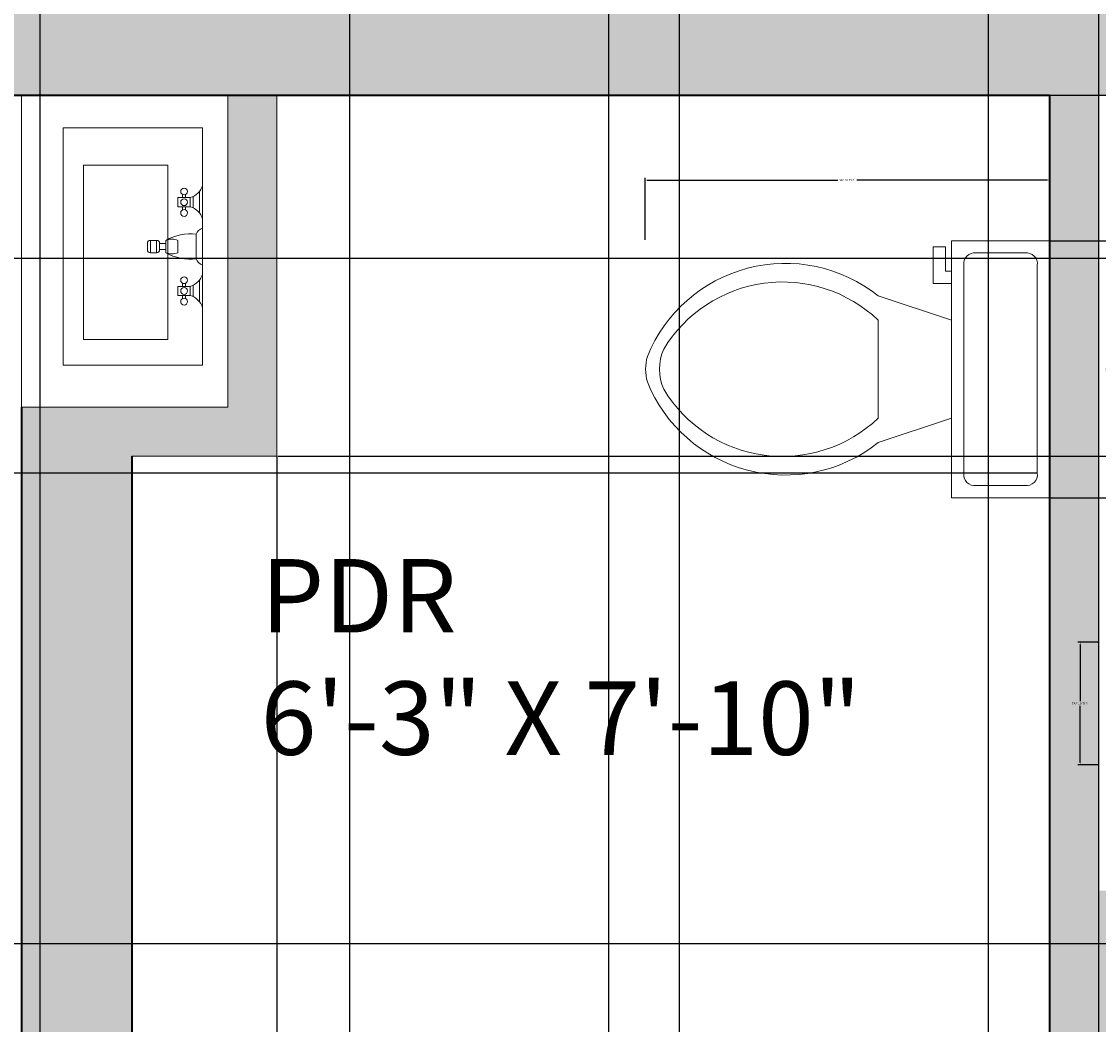
# Model space of a CAD drawing. Units: inches. Extents: x 818 to 1898, y 976 to 2364.
# Tile 51 of 96: x 1512 to 1600, y 1791 to 1873. Entities that reach past the tile are written whole.
import ezdxf

# ---------------------------------------------------------------- set-up
doc = ezdxf.new("R2010")
doc.units = ezdxf.units.IN
doc.header["$LTSCALE"] = 5
doc.header["$MEASUREMENT"] = 0
for name, color, linetype, lineweight in [('A-ANNO-DIMS', 2, 'Continuous', 18), ('A-AREA-IDEN', 7, 'Continuous', 18), ('A-FLOR-FIXT', 9, 'Continuous', 18), ('A-WALL', 7, 'Continuous', 40)]:
    doc.layers.add(name, color=color, linetype=linetype, lineweight=lineweight)
doc.layers.add('A-WALL-PATT', color=251, linetype='Continuous', lineweight=13, true_color=0x636466)
doc.styles.get("Standard").update_dxf_attribs({"font": 'arial.ttf'})
doc.dimstyles.get("Standard").update_dxf_attribs({"dimtxt": 0.18, "dimasz": 0.18, "dimexe": 0.18, "dimexo": 0.0625, "dimgap": 0.09, "dimtad": 0, "dimtih": 1, "dimtoh": 1, "dimdec": 4, "dimzin": 0, "dimdsep": 46, "dimtxsty": 'Standard', "dimcen": 0.09, "dimadec": 0, "dimazin": 0, "dimtfac": 1, "dimtdec": 4, "dimtofl": 0, "dimtmove": 0, "dimatfit": 3, "dimfxl": 1, "dimtolj": 1, "dimtzin": 0, "dimarcsym": 0})

# ---------------------------------------------------------------- blocks, each defined once
blk = doc.blocks.new('Toilet - top')
for p, q in [((9.5, -6), (9.5, -2)), ((-10, -8.5), (-8, -8.5)), ((-10, -9.5), (-10, -8.5)), ((-8, -8.5), (-8, -8)), ((-7, -8), (-7, -9.5)), ((-4, -8), (-6, -14)), ((4, -8), (6, -14)), ((-7, -9.5), (-10, -9.5)), ((4, -14), (-4, -14))]:
    blk.add_line(p, q)
blk.add_lwpolyline([(10.5, -8), (10.5, 0), (-10.5, 0), (-10.5, -8)], close=True)
for points in [[(8.5, -1), (-8.5, -1)], [(-9.5, -2), (-9.5, -6)], [(-8.5, -7), (8.5, -7)]]:
    blk.add_lwpolyline(points)
for centre, radius, start, end in [((-8.625, -1.875), 0.884, 81.8699, 188.1301), ((8.625, -1.875), 0.884, 351.8699, 98.1301), ((-8.625, -6.125), 0.884, 171.8699, 278.1301), ((8.625, -6.125), 0.884, 261.8699, 8.1301), ((3.52, -21.58), 12.169, 141.46911, 247.97143), ((4.2, -21.817), 11.329, 136.36773, 238.94682), ((-3.519, -21.58), 12.169, 292.02843, 38.53071), ((-4.2, -21.817), 11.329, 301.05301, 43.63209), ((0, -27.876), 4, 245.73182, 294.26817), ((0, -29), 4, 254.86053, 285.13947)]:
    blk.add_arc(centre, radius, start, end)
blk = doc.blocks.new('Faucet - Bathroom front')
for p, q in [((-0.5, 4.25), (0.5, 4.25)), ((0.5, 3.75), (-0.5, 3.75)), ((-0.5, 3), (0.5, 3)), ((-0.25, 3), (-0.25, 3.5)), ((0.25, 3.5), (0.25, 3)), ((0.5, 2), (-0.5, 2)), ((-4, 1.625), (-4.25, 1.625)), ((-4, 1.375), (-4.25, 1.375)), ((-3.25, 1.625), (-3, 1.625)), ((-3.25, 1.375), (-3, 1.375)), ((3.25, 1.625), (3, 1.625)), ((3.25, 1.375), (3, 1.375)), ((4, 1.625), (4.25, 1.625)), ((4, 1.375), (4.25, 1.375)), ((-5, 0), (-2.25, 0)), ((-4.5087, 0.25), (-2.7408, 0.25)), ((-3.1442, 0.75), (-4.0979, 0.75)), ((-1.5, 0), (1.5, 0)), ((-1, 0.5), (1, 0.5)), ((2.25, 0), (5, 0)), ((2.7413, 0.25), (4.5092, 0.25)), ((4.1058, 0.75), (3.1521, 0.75))]:
    blk.add_line(p, q)
for points in [[(-0.25, 4.5), (0.25, 4.5)], [(-0.5, 3.75), (-0.5, 4.25)], [(0.5, 4.25), (0.5, 3.75)], [(0.25, 3.5), (-0.25, 3.5)]]:
    blk.add_lwpolyline(points)
for points in [[(-4, 1), (-4, 2), (-3.25, 2), (-3.25, 1)], [(3.25, 1), (3.25, 2), (4, 2), (4, 1)]]:
    blk.add_lwpolyline(points, close=True)
for centre in [(-4.5, 1.5), (-3.625, 1.5), (-2.75, 1.5), (2.75, 1.5), (3.625, 1.5), (4.5, 1.5)]:
    blk.add_circle(centre, 0.2795)
for centre, radius, start, end in [((-0.2575, 4.2575), 0.2426, 88.22243, 181.7776), ((0.2575, 4.2575), 0.2426, 358.2224, 91.77757), ((-0.2575, 3.7425), 0.2426, 178.2224, 271.7776), ((0.2575, 3.7425), 0.2426, 268.2224, 1.777565), ((3, 1), 4.0311, 150.2551, 187.125), ((0.6413, 2.5), 1.246, 156.3417, 203.6583), ((-3, 1), 4.0311, 352.875, 29.74488), ((-0.6413, 2.5), 1.246, 336.3417, 23.65835), ((-5.375, 1.375), 1.4252, 285.2551, 344.7449), ((-1.875, 1.375), 1.4252, 195.2551, 254.7449), ((1.875, 1.375), 1.4252, 285.2551, 344.7449), ((5.375, 1.375), 1.4252, 195.2551, 254.7449), ((-0.7962, -0.2038), 0.7327, 106.1502, 163.8498), ((0.7962, -0.2038), 0.7327, 16.1502, 73.84979)]:
    blk.add_arc(centre, radius, start, end)
blk = doc.blocks.new('*D36')
at = {"layer": 'A-ANNO-DIMS', "color": 0, "lineweight": -2, "ltscale": 5, "transparency": 16777216}
for p, q in [((1599.663, 1822.366), (1598.045, 1822.366)), ((1598.225, 1822.186), (1598.225, 1817.548)), ((1598.225, 1812.546), (1598.225, 1817.184)), ((1599.663, 1812.366), (1598.045, 1812.366))]:
    blk.add_line(p, q, dxfattribs=at)
at = {"layer": 'A-ANNO-DIMS', "color": 0, "ltscale": 5, "transparency": 16777216}
for points in [[(1598.195, 1822.186), (1598.255, 1822.186), (1598.225, 1822.366)], [(1598.195, 1812.546), (1598.255, 1812.546), (1598.225, 1812.366)]]:
    blk.add_solid(points, dxfattribs=at)
at = {"layer": 'Defpoints', "color": 0, "ltscale": 5, "transparency": 16777216}
for p in [(1599.725, 1822.366), (1598.225, 1812.366), (1599.725, 1812.366)]:
    blk.add_point(p, dxfattribs=at)
at = {"layer": 'A-ANNO-DIMS', "color": 0, "ltscale": 5, "transparency": 16777216, "insert": (1598.225, 1817.366), "char_height": 0.18, "attachment_point": 5}
blk.add_mtext('\\A1;TAP 10 TYP.', dxfattribs=at)
blk = doc.blocks.new('*D40')
at = {"layer": 'A-ANNO-DIMS', "color": 0, "lineweight": -2, "ltscale": 5, "transparency": 16777216}
for p, q in [((1562.679, 1855.247), (1562.679, 1860.321)), ((1595.725, 1855.247), (1595.725, 1860.321)), ((1562.859, 1860.141), (1578.426, 1860.141)), ((1595.545, 1860.141), (1579.978, 1860.141))]:
    blk.add_line(p, q, dxfattribs=at)
at = {"layer": 'A-ANNO-DIMS', "color": 0, "ltscale": 5, "transparency": 16777216}
for points in [[(1562.859, 1860.171), (1562.859, 1860.111), (1562.679, 1860.141)], [(1595.545, 1860.171), (1595.545, 1860.111), (1595.725, 1860.141)]]:
    blk.add_solid(points, dxfattribs=at)
at = {"layer": 'Defpoints', "color": 0, "ltscale": 5, "transparency": 16777216}
for p in [(1595.725, 1860.141), (1562.679, 1855.184), (1595.725, 1855.184)]:
    blk.add_point(p, dxfattribs=at)
at = {"layer": 'A-ANNO-DIMS', "color": 0, "ltscale": 5, "transparency": 16777216, "insert": (1579.202, 1860.141), "char_height": 0.18, "attachment_point": 5}
blk.add_mtext('\\A1;WC 33 TYP.', dxfattribs=at)
blk = doc.blocks.new('*D41')
at = {"layer": 'A-ANNO-DIMS', "color": 0, "lineweight": -2, "ltscale": 5, "transparency": 16777216}
for p, q in [((1595.788, 1855.184), (1600.862, 1855.184)), ((1600.682, 1855.004), (1600.682, 1844.865)), ((1600.682, 1834.364), (1600.682, 1844.504)), ((1595.788, 1834.184), (1600.862, 1834.184))]:
    blk.add_line(p, q, dxfattribs=at)
at = {"layer": 'A-ANNO-DIMS', "color": 0, "ltscale": 5, "transparency": 16777216}
for points in [[(1600.652, 1855.004), (1600.712, 1855.004), (1600.682, 1855.184)], [(1600.652, 1834.364), (1600.712, 1834.364), (1600.682, 1834.184)]]:
    blk.add_solid(points, dxfattribs=at)
at = {"layer": 'Defpoints', "color": 0, "ltscale": 5, "transparency": 16777216}
for p in [(1595.725, 1855.184), (1595.725, 1834.184), (1600.682, 1834.184)]:
    blk.add_point(p, dxfattribs=at)
at = {"layer": 'A-ANNO-DIMS', "color": 0, "ltscale": 5, "transparency": 16777216, "insert": (1600.682, 1844.684), "char_height": 0.18, "attachment_point": 5}
blk.add_mtext('\\A1;21 TYP.', dxfattribs=at)
blk = doc.blocks.new('*D85')
at = {"layer": 'A-ANNO-DIMS', "color": 0, "lineweight": -2, "ltscale": 5, "transparency": 16777216}
for p, q in [((1258.788, 2053.078), (1897.916, 2053.078)), ((1897.736, 2052.898), (1897.736, 1876.76)), ((1897.736, 1700.258), (1897.736, 1876.396)), ((1258.788, 1700.078), (1897.916, 1700.078))]:
    blk.add_line(p, q, dxfattribs=at)
at = {"layer": 'A-ANNO-DIMS', "color": 0, "ltscale": 5, "transparency": 16777216}
for points in [[(1897.706, 2052.898), (1897.766, 2052.898), (1897.736, 2053.078)], [(1897.706, 1700.258), (1897.766, 1700.258), (1897.736, 1700.078)]]:
    blk.add_solid(points, dxfattribs=at)
at = {"layer": 'Defpoints', "color": 0, "ltscale": 5, "transparency": 16777216}
for p in [(1258.725, 2053.078), (1897.736, 2053.078), (1258.725, 1700.078)]:
    blk.add_point(p, dxfattribs=at)
at = {"layer": 'A-ANNO-DIMS', "color": 0, "ltscale": 5, "transparency": 16777216, "insert": (1897.736, 1876.578), "char_height": 0.18, "attachment_point": 5}
blk.add_mtext('\\A1;353', dxfattribs=at)
blk = doc.blocks.new('*D101')
at = {"layer": 'A-ANNO-DIMS', "color": 0, "lineweight": -2, "ltscale": 5, "transparency": 16777216}
for p, q in [((1507.298, 1071.118), (1507.298, 2363.873)), ((1507.478, 2363.693), (1535.997, 2363.693)), ((1565.303, 2363.693), (1536.785, 2363.693)), ((1565.483, 1071.118), (1565.483, 2363.873))]:
    blk.add_line(p, q, dxfattribs=at)
at = {"layer": 'A-ANNO-DIMS', "color": 0, "ltscale": 5, "transparency": 16777216}
for points in [[(1507.478, 2363.723), (1507.478, 2363.663), (1507.298, 2363.693)], [(1565.303, 2363.723), (1565.303, 2363.663), (1565.483, 2363.693)]]:
    blk.add_solid(points, dxfattribs=at)
at = {"layer": 'Defpoints', "color": 0, "ltscale": 5, "transparency": 16777216}
for p in [(1565.483, 2363.693), (1507.298, 1071.055), (1565.483, 1071.055)]:
    blk.add_point(p, dxfattribs=at)
at = {"layer": 'A-ANNO-DIMS', "color": 0, "ltscale": 5, "transparency": 16777216, "insert": (1536.391, 2363.693), "char_height": 0.18, "attachment_point": 5}
blk.add_mtext('\\A1;58.19', dxfattribs=at)
blk = doc.blocks.new('*D102')
at = {"layer": 'A-ANNO-DIMS', "color": 0, "lineweight": -2, "ltscale": 5, "transparency": 16777216}
for p, q in [((1565.483, 1071.118), (1565.483, 2363.873)), ((1565.663, 2363.693), (1595.635, 2363.693)), ((1626.395, 2363.693), (1596.423, 2363.693)), ((1626.575, 1071.118), (1626.575, 2363.873))]:
    blk.add_line(p, q, dxfattribs=at)
at = {"layer": 'A-ANNO-DIMS', "color": 0, "ltscale": 5, "transparency": 16777216}
for points in [[(1565.663, 2363.723), (1565.663, 2363.663), (1565.483, 2363.693)], [(1626.395, 2363.723), (1626.395, 2363.663), (1626.575, 2363.693)]]:
    blk.add_solid(points, dxfattribs=at)
at = {"layer": 'Defpoints', "color": 0, "ltscale": 5, "transparency": 16777216}
for p in [(1626.575, 2363.693), (1565.483, 1071.055), (1626.575, 1071.055)]:
    blk.add_point(p, dxfattribs=at)
at = {"layer": 'A-ANNO-DIMS', "color": 0, "ltscale": 5, "transparency": 16777216, "insert": (1596.029, 2363.693), "char_height": 0.18, "attachment_point": 5}
blk.add_mtext('\\A1;61.09', dxfattribs=at)
blk = doc.blocks.new('*D120')
at = {"layer": 'A-ANNO-DIMS', "color": 0, "lineweight": -2, "ltscale": 5, "transparency": 16777216}
for p, q in [((1766.29, 1797.717), (818.026, 1797.717)), ((818.206, 1797.537), (818.206, 1757.534)), ((818.206, 1717.167), (818.206, 1757.17)), ((1766.29, 1716.987), (818.026, 1716.987))]:
    blk.add_line(p, q, dxfattribs=at)
at = {"layer": 'A-ANNO-DIMS', "color": 0, "ltscale": 5, "transparency": 16777216}
for points in [[(818.176, 1797.537), (818.236, 1797.537), (818.206, 1797.717)], [(818.176, 1717.167), (818.236, 1717.167), (818.206, 1716.987)]]:
    blk.add_solid(points, dxfattribs=at)
at = {"layer": 'Defpoints', "color": 0, "ltscale": 5, "transparency": 16777216}
for p in [(818.206, 1797.717), (1766.352, 1797.717), (1766.352, 1716.987)]:
    blk.add_point(p, dxfattribs=at)
at = {"layer": 'A-ANNO-DIMS', "color": 0, "ltscale": 5, "transparency": 16777216, "insert": (818.206, 1757.352), "char_height": 0.18, "attachment_point": 5}
blk.add_mtext('\\A1;80.73', dxfattribs=at)
blk = doc.blocks.new('*D121')
at = {"layer": 'A-ANNO-DIMS', "color": 0, "lineweight": -2, "ltscale": 5, "transparency": 16777216}
for p, q in [((1766.29, 1884.203), (818.026, 1884.203)), ((818.206, 1884.023), (818.206, 1841.142)), ((818.206, 1797.897), (818.206, 1840.778)), ((1766.29, 1797.717), (818.026, 1797.717))]:
    blk.add_line(p, q, dxfattribs=at)
at = {"layer": 'A-ANNO-DIMS', "color": 0, "ltscale": 5, "transparency": 16777216}
for points in [[(818.176, 1884.023), (818.236, 1884.023), (818.206, 1884.203)], [(818.176, 1797.897), (818.236, 1797.897), (818.206, 1797.717)]]:
    blk.add_solid(points, dxfattribs=at)
at = {"layer": 'Defpoints', "color": 0, "ltscale": 5, "transparency": 16777216}
for p in [(818.206, 1884.203), (1766.352, 1884.203), (1766.352, 1797.717)]:
    blk.add_point(p, dxfattribs=at)
at = {"layer": 'A-ANNO-DIMS', "color": 0, "ltscale": 5, "transparency": 16777216, "insert": (818.206, 1840.96), "char_height": 0.18, "attachment_point": 5}
blk.add_mtext('\\A1;86.49', dxfattribs=at)
blk = doc.blocks.new('*D175')
at = {"layer": 'A-ANNO-DIMS', "color": 0, "lineweight": -2, "ltscale": 5, "transparency": 16777216}
for p, q in [((1559.725, 1647.641), (1559.725, 2363.873)), ((1559.905, 2363.693), (1614.445, 2363.693)), ((1669.545, 2363.693), (1615.005, 2363.693)), ((1669.725, 1647.641), (1669.725, 2363.873))]:
    blk.add_line(p, q, dxfattribs=at)
at = {"layer": 'A-ANNO-DIMS', "color": 0, "ltscale": 5, "transparency": 16777216}
for points in [[(1559.905, 2363.723), (1559.905, 2363.663), (1559.725, 2363.693)], [(1669.545, 2363.723), (1669.545, 2363.663), (1669.725, 2363.693)]]:
    blk.add_solid(points, dxfattribs=at)
at = {"layer": 'Defpoints', "color": 0, "ltscale": 5, "transparency": 16777216}
for p in [(1669.725, 2363.693), (1559.725, 1647.578), (1669.725, 1647.578)]:
    blk.add_point(p, dxfattribs=at)
at = {"layer": 'A-ANNO-DIMS', "color": 0, "ltscale": 5, "transparency": 16777216, "insert": (1614.725, 2363.693), "char_height": 0.18, "attachment_point": 5}
blk.add_mtext('\\A1;110', dxfattribs=at)
blk = doc.blocks.new('*D215')
at = {"layer": 'A-ANNO-DIMS', "color": 0, "lineweight": -2, "ltscale": 5, "transparency": 16777216}
for p, q in [((1590.663, 1876.078), (818.026, 1876.078)), ((818.206, 1875.898), (818.206, 1781.76)), ((818.206, 1687.258), (818.206, 1781.396)), ((1511.663, 1687.078), (818.026, 1687.078))]:
    blk.add_line(p, q, dxfattribs=at)
at = {"layer": 'A-ANNO-DIMS', "color": 0, "ltscale": 5, "transparency": 16777216}
for points in [[(818.176, 1875.898), (818.236, 1875.898), (818.206, 1876.078)], [(818.176, 1687.258), (818.236, 1687.258), (818.206, 1687.078)]]:
    blk.add_solid(points, dxfattribs=at)
at = {"layer": 'Defpoints', "color": 0, "ltscale": 5, "transparency": 16777216}
for p in [(818.206, 1876.078), (1590.725, 1876.078), (1511.725, 1687.078)]:
    blk.add_point(p, dxfattribs=at)
at = {"layer": 'A-ANNO-DIMS', "color": 0, "ltscale": 5, "transparency": 16777216, "insert": (818.206, 1781.578), "char_height": 0.18, "attachment_point": 5}
blk.add_mtext('\\A1;189', dxfattribs=at)
blk = doc.blocks.new('*D224')
at = {"layer": 'A-ANNO-DIMS', "color": 0, "lineweight": -2, "ltscale": 5, "transparency": 16777216}
for p, q in [((1520.725, 1837.52), (1520.725, 975.663)), ((1532.593, 1837.52), (1532.593, 975.663)), ((1520.905, 975.843), (1526.204, 975.843)), ((1532.413, 975.843), (1527.114, 975.843))]:
    blk.add_line(p, q, dxfattribs=at)
at = {"layer": 'A-ANNO-DIMS', "color": 0, "ltscale": 5, "transparency": 16777216}
for points in [[(1520.905, 975.873), (1520.905, 975.813), (1520.725, 975.843)], [(1532.413, 975.873), (1532.413, 975.813), (1532.593, 975.843)]]:
    blk.add_solid(points, dxfattribs=at)
at = {"layer": 'Defpoints', "color": 0, "ltscale": 5, "transparency": 16777216}
for p in [(1520.725, 1837.582), (1532.593, 1837.582), (1532.593, 975.843)]:
    blk.add_point(p, dxfattribs=at)
at = {"layer": 'A-ANNO-DIMS', "color": 0, "ltscale": 5, "transparency": 16777216, "insert": (1526.659, 975.843), "char_height": 0.18, "attachment_point": 5}
blk.add_mtext('\\A1;11.868', dxfattribs=at)
blk = doc.blocks.new('*D225')
at = {"layer": 'A-ANNO-DIMS', "color": 0, "lineweight": -2, "ltscale": 5, "transparency": 16777216}
for p, q in [((1532.655, 1867.078), (1897.916, 1867.078)), ((1897.736, 1866.898), (1897.736, 1852.512)), ((1897.736, 1837.762), (1897.736, 1852.148)), ((1532.655, 1837.582), (1897.916, 1837.582))]:
    blk.add_line(p, q, dxfattribs=at)
at = {"layer": 'A-ANNO-DIMS', "color": 0, "ltscale": 5, "transparency": 16777216}
for points in [[(1897.706, 1866.898), (1897.766, 1866.898), (1897.736, 1867.078)], [(1897.706, 1837.762), (1897.766, 1837.762), (1897.736, 1837.582)]]:
    blk.add_solid(points, dxfattribs=at)
at = {"layer": 'Defpoints', "color": 0, "ltscale": 5, "transparency": 16777216}
for p in [(1532.593, 1867.078), (1897.736, 1867.078), (1532.593, 1837.582)]:
    blk.add_point(p, dxfattribs=at)
at = {"layer": 'A-ANNO-DIMS', "color": 0, "ltscale": 5, "transparency": 16777216, "insert": (1897.736, 1852.33), "char_height": 0.18, "attachment_point": 5}
blk.add_mtext('\\A1;29.496', dxfattribs=at)
blk = doc.blocks.new('*D227')
at = {"layer": 'A-ANNO-DIMS', "color": 0, "lineweight": -2, "ltscale": 5, "transparency": 16777216}
for p, q in [((1595.663, 1867.078), (818.026, 1867.078)), ((818.206, 1866.898), (818.206, 1851.813)), ((818.206, 1836.364), (818.206, 1851.449)), ((1594.663, 1836.184), (818.026, 1836.184))]:
    blk.add_line(p, q, dxfattribs=at)
at = {"layer": 'A-ANNO-DIMS', "color": 0, "ltscale": 5, "transparency": 16777216}
for points in [[(818.176, 1866.898), (818.236, 1866.898), (818.206, 1867.078)], [(818.176, 1836.364), (818.236, 1836.364), (818.206, 1836.184)]]:
    blk.add_solid(points, dxfattribs=at)
at = {"layer": 'Defpoints', "color": 0, "ltscale": 5, "transparency": 16777216}
for p in [(818.206, 1867.078), (1595.725, 1867.078), (1594.725, 1836.184)]:
    blk.add_point(p, dxfattribs=at)
at = {"layer": 'A-ANNO-DIMS', "color": 0, "ltscale": 5, "transparency": 16777216, "insert": (818.206, 1851.631), "char_height": 0.18, "attachment_point": 5}
blk.add_mtext('\\A1;30.894', dxfattribs=at)
blk = doc.blocks.new('*D229')
at = {"layer": 'A-ANNO-DIMS', "color": 0, "lineweight": -2, "ltscale": 5, "transparency": 16777216}
for p, q in [((1599.725, 2044.016), (1599.725, 975.663)), ((1620.142, 2036.056), (1620.142, 975.663)), ((1599.905, 975.843), (1609.468, 975.843)), ((1619.962, 975.843), (1610.398, 975.843))]:
    blk.add_line(p, q, dxfattribs=at)
at = {"layer": 'A-ANNO-DIMS', "color": 0, "ltscale": 5, "transparency": 16777216}
for points in [[(1599.905, 975.873), (1599.905, 975.813), (1599.725, 975.843)], [(1619.962, 975.873), (1619.962, 975.813), (1620.142, 975.843)]]:
    blk.add_solid(points, dxfattribs=at)
at = {"layer": 'Defpoints', "color": 0, "ltscale": 5, "transparency": 16777216}
for p in [(1599.725, 2044.078), (1620.142, 2036.118), (1620.142, 975.843)]:
    blk.add_point(p, dxfattribs=at)
at = {"layer": 'A-ANNO-DIMS', "color": 0, "ltscale": 5, "transparency": 16777216, "insert": (1609.933, 975.843), "char_height": 0.18, "attachment_point": 5}
blk.add_mtext('\\A1;20.416', dxfattribs=at)
blk = doc.blocks.new('*D242')
at = {"layer": 'A-ANNO-DIMS', "color": 0, "lineweight": -2, "ltscale": 5, "transparency": 16777216}
for p, q in [((1488.259, 1948.598), (1488.259, 975.663)), ((1513.231, 1948.598), (1513.231, 975.663)), ((1488.439, 975.843), (1500.349, 975.843)), ((1513.051, 975.843), (1501.14, 975.843))]:
    blk.add_line(p, q, dxfattribs=at)
at = {"layer": 'A-ANNO-DIMS', "color": 0, "ltscale": 5, "transparency": 16777216}
for points in [[(1488.439, 975.873), (1488.439, 975.813), (1488.259, 975.843)], [(1513.051, 975.873), (1513.051, 975.813), (1513.231, 975.843)]]:
    blk.add_solid(points, dxfattribs=at)
at = {"layer": 'Defpoints', "color": 0, "ltscale": 5, "transparency": 16777216}
for p in [(1488.259, 1948.66), (1513.231, 1948.66), (1513.231, 975.843)]:
    blk.add_point(p, dxfattribs=at)
at = {"layer": 'A-ANNO-DIMS', "color": 0, "ltscale": 5, "transparency": 16777216, "insert": (1500.745, 975.843), "char_height": 0.18, "attachment_point": 5}
blk.add_mtext('\\A1;24.97', dxfattribs=at)
blk = doc.blocks.new('*D243')
at = {"layer": 'A-ANNO-DIMS', "color": 0, "lineweight": -2, "ltscale": 5, "transparency": 16777216}
for p, q in [((1451.77, 2020.016), (1451.77, 975.663)), ((1590.725, 2020.016), (1590.725, 975.663)), ((1451.95, 975.843), (1520.792, 975.843)), ((1590.545, 975.843), (1521.703, 975.843))]:
    blk.add_line(p, q, dxfattribs=at)
at = {"layer": 'A-ANNO-DIMS', "color": 0, "ltscale": 5, "transparency": 16777216}
for points in [[(1451.95, 975.873), (1451.95, 975.813), (1451.77, 975.843)], [(1590.545, 975.873), (1590.545, 975.813), (1590.725, 975.843)]]:
    blk.add_solid(points, dxfattribs=at)
at = {"layer": 'Defpoints', "color": 0, "ltscale": 5, "transparency": 16777216}
for p in [(1451.77, 2020.078), (1590.725, 2020.078), (1590.725, 975.843)]:
    blk.add_point(p, dxfattribs=at)
at = {"layer": 'A-ANNO-DIMS', "color": 0, "ltscale": 5, "transparency": 16777216, "insert": (1521.247, 975.843), "char_height": 0.18, "attachment_point": 5}
blk.add_mtext('\\A1;138.96', dxfattribs=at)
blk = doc.blocks.new('*D253')
at = {"layer": 'A-ANNO-DIMS', "color": 0, "lineweight": -2, "ltscale": 5, "transparency": 16777216}
for p, q in [((1485.122, 2053.016), (1485.122, 975.663)), ((1538.516, 2053.016), (1538.516, 975.663)), ((1485.302, 975.843), (1511.425, 975.843)), ((1538.336, 975.843), (1512.212, 975.843))]:
    blk.add_line(p, q, dxfattribs=at)
at = {"layer": 'A-ANNO-DIMS', "color": 0, "ltscale": 5, "transparency": 16777216}
for points in [[(1485.302, 975.873), (1485.302, 975.813), (1485.122, 975.843)], [(1538.336, 975.873), (1538.336, 975.813), (1538.516, 975.843)]]:
    blk.add_solid(points, dxfattribs=at)
at = {"layer": 'Defpoints', "color": 0, "ltscale": 5, "transparency": 16777216}
for p in [(1485.122, 2053.078), (1538.516, 2053.078), (1538.516, 975.843)]:
    blk.add_point(p, dxfattribs=at)
at = {"layer": 'A-ANNO-DIMS', "color": 0, "ltscale": 5, "transparency": 16777216, "insert": (1511.819, 975.843), "char_height": 0.18, "attachment_point": 5}
blk.add_mtext('\\A1;53.39', dxfattribs=at)
blk = doc.blocks.new('*D275')
at = {"layer": 'A-ANNO-DIMS', "color": 0, "lineweight": -2, "ltscale": 5, "transparency": 16777216}
for p, q in [((1377.842, 1897.866), (1897.916, 1897.866)), ((1897.736, 1897.686), (1897.736, 1875.988)), ((1897.736, 1853.93), (1897.736, 1875.628)), ((1377.842, 1853.75), (1897.916, 1853.75))]:
    blk.add_line(p, q, dxfattribs=at)
at = {"layer": 'A-ANNO-DIMS', "color": 0, "ltscale": 5, "transparency": 16777216}
for points in [[(1897.706, 1897.686), (1897.766, 1897.686), (1897.736, 1897.866)], [(1897.706, 1853.93), (1897.766, 1853.93), (1897.736, 1853.75)]]:
    blk.add_solid(points, dxfattribs=at)
at = {"layer": 'Defpoints', "color": 0, "ltscale": 5, "transparency": 16777216}
for p in [(1377.779, 1897.866), (1897.736, 1897.866), (1377.779, 1853.75)]:
    blk.add_point(p, dxfattribs=at)
at = {"layer": 'A-ANNO-DIMS', "color": 0, "ltscale": 5, "transparency": 16777216, "insert": (1897.736, 1875.808), "char_height": 0.18, "attachment_point": 5}
blk.add_mtext('\\A1;44.12', dxfattribs=at)
blk = doc.blocks.new('*D282')
at = {"layer": 'A-ANNO-DIMS', "color": 0, "lineweight": -2, "ltscale": 5, "transparency": 16777216}
for p, q in [((1422.083, 2081.188), (1897.916, 2081.188)), ((1897.736, 2081.008), (1897.736, 1884.315)), ((1897.736, 1687.258), (1897.736, 1883.951)), ((1463.788, 1687.078), (1897.916, 1687.078))]:
    blk.add_line(p, q, dxfattribs=at)
at = {"layer": 'A-ANNO-DIMS', "color": 0, "ltscale": 5, "transparency": 16777216}
for points in [[(1897.706, 2081.008), (1897.766, 2081.008), (1897.736, 2081.188)], [(1897.706, 1687.258), (1897.766, 1687.258), (1897.736, 1687.078)]]:
    blk.add_solid(points, dxfattribs=at)
at = {"layer": 'Defpoints', "color": 0, "ltscale": 5, "transparency": 16777216}
for p in [(1422.02, 2081.188), (1897.736, 2081.188), (1463.725, 1687.078)]:
    blk.add_point(p, dxfattribs=at)
at = {"layer": 'A-ANNO-DIMS', "color": 0, "ltscale": 5, "transparency": 16777216, "insert": (1897.736, 1884.133), "char_height": 0.18, "attachment_point": 5}
blk.add_mtext('\\A1;394.1', dxfattribs=at)

msp = doc.modelspace()

# ---------------------------------------------------------------- hatches: boundary and pattern name
at = {"layer": 'A-WALL-PATT', "ltscale": 5}
h = msp.add_hatch(color=256, dxfattribs=at)
h.dxf.hatch_style = 1
h.paths.add_polyline_path([(1267.7252, 1928.9218), (1258.7251, 1928.9218), (1258.7251, 1913.6401), (1250.3029, 1913.6401), (1250.3029, 1878.3919), (1258.7251, 1878.3919), (1258.7251, 1862.9652), (1267.7252, 1862.9652)])
h.paths.add_polyline_path([(1267.7252, 1814.9652), (1258.7251, 1814.9652), (1258.7251, 1755.3321), (1267.7252, 1755.3321)])
h.paths.add_polyline_path([(1463.7251, 1696.0782), (1267.7252, 1696.0782), (1267.7252, 1707.3321), (1258.7251, 1707.3321), (1258.7251, 1700.0782), (1251.9333, 1700.0782), (1251.9333, 1687.0782), (1463.7251, 1687.0782)])
h.paths.add_polyline_path([(1714.7252, 1717.3178), (1705.7252, 1717.3178), (1705.7252, 1696.0782), (1599.7251, 1696.0782), (1599.7251, 1790.0782), (1705.7252, 1790.0782), (1705.7252, 1785.6125), (1714.7252, 1785.6125), (1714.7252, 1827.2125), (1705.7252, 1827.2125), (1705.7252, 1802.0782), (1599.7251, 1802.0782), (1599.7251, 1867.0782), (1705.7252, 1867.0782), (1705.7252, 1857.2125), (1714.7252, 1857.2125), (1714.7252, 1930.0316), (1741.8409, 1930.0316), (1741.8409, 1935.0316), (1714.7252, 1935.0316), (1714.7252, 1957.0338), (1741.8409, 1957.0338), (1741.8409, 1962.0338), (1714.7252, 1962.0338), (1705.7252, 1962.0338), (1705.7252, 1948.0782), (1599.7251, 1948.0782), (1599.7251, 1981.0782), (1590.7251, 1981.0782), (1590.7251, 1941.0782), (1620.7252, 1941.0782), (1705.7252, 1941.0782), (1705.7252, 1876.0782), (1599.7251, 1876.0782), (1599.7251, 1911.0782), (1590.7251, 1911.0782), (1590.7251, 1876.0782), (1429.2252, 1876.0782), (1429.2252, 1867.0782), (1511.7251, 1867.0782), (1528.593, 1867.0782), (1595.7251, 1867.0782), (1595.7251, 1773.0782), (1520.7251, 1773.0782), (1520.7251, 1837.5823), (1532.593, 1837.5823), (1532.593, 1867.0782), (1528.593, 1867.0782), (1528.593, 1841.5823), (1511.7251, 1841.5823), (1511.7251, 1744.9714), (1520.7251, 1744.9714), (1520.7251, 1761.0782), (1595.7251, 1761.0782), (1595.7251, 1696.0782), (1520.7251, 1696.0782), (1520.7251, 1716.0454), (1511.7251, 1716.0454), (1511.7251, 1696.0782), (1511.7251, 1687.0782), (1714.7252, 1687.0782)])
h.paths.add_polyline_path([(1714.7252, 2053.0782), (1714.7252, 2081.1881), (1709.7252, 2081.1881), (1709.7252, 2053.0782), (1681.6446, 2053.0782), (1681.6446, 2081.1881), (1676.6446, 2081.1881), (1676.6446, 2053.0782), (1538.5155, 2053.0782), (1538.5155, 2044.0782), (1590.7251, 2044.0782), (1590.7251, 2011.0782), (1599.7251, 2011.0782), (1599.7251, 2044.0782), (1705.7252, 2044.0782), (1705.7252, 2014.5114), (1714.7252, 2014.5114)])
h.paths.add_polyline_path([(1485.1216, 2053.0782), (1422.02, 2053.0782), (1422.02, 2081.1881), (1413.02, 2081.1881), (1413.02, 2053.0782), (1399.6356, 2053.0782), (1399.6356, 2081.1881), (1390.6356, 2081.1881), (1390.6356, 2053.0782), (1388.0315, 2053.0782), (1388.0315, 2044.0782), (1416.2743, 2044.0782), (1485.1216, 2044.0782)])
h.paths.add_polyline_path([(1330.305, 2053.0782), (1258.7251, 2053.0782), (1258.7251, 2019.2871), (1267.7252, 2019.2871), (1267.7252, 2044.0782), (1330.305, 2044.0782)])
h.paths.add_polyline_path([(1258.7251, 2053.0782), (1214.6577, 2053.0782), (1214.6577, 2044.0782), (1258.7251, 2044.0782)])
h.paths.add_polyline_path([(1214.6577, 2053.0782), (1180.349, 2053.0782), (1180.349, 2044.0782), (1214.6577, 2044.0782)])
h.paths.add_polyline_path([(1714.7252, 1639.5782), (1741.8409, 1639.5782), (1741.8409, 1643.5782), (1714.7252, 1643.5782), (1714.7252, 1649.9029), (1705.7252, 1649.9029), (1705.7252, 1600.0782), (1477.7252, 1600.0782), (1477.7252, 1591.0782), (1520.7251, 1591.0782), (1616.7252, 1591.0782), (1616.7252, 1416.6857), (1622.7252, 1416.6857), (1622.7252, 1463.0782), (1624.7252, 1463.0782), (1624.7252, 1467.0782), (1622.7252, 1467.0782), (1622.7252, 1591.0782), (1705.7252, 1591.0782), (1705.7252, 1545.0782), (1714.7252, 1545.0782), (1741.8409, 1545.0782), (1741.8409, 1549.0782), (1714.7252, 1549.0782), (1714.7252, 1593.9175), (1737.8409, 1593.9175), (1737.8409, 1597.9175), (1714.7252, 1597.9175)])
h.paths.add_polyline_path([(1674.9024, 2060.7419), (1714.7045, 2060.7419), (1714.7045, 2073.1061), (1674.9024, 2073.1061)], flags=25)
h.paths.add_polyline_path([(1394.5468, 2061.6618), (1422.2344, 2061.6618), (1422.2344, 2074.0261), (1394.5468, 2074.0261)], flags=24)

# ---------------------------------------------------------------- linework, layer by layer
at = {"layer": 'A-FLOR-FIXT'}
for p, q in [((1528.593, 1867.0782), (1528.593, 1841.5823)), ((1532.593, 1867.0782), (1532.593, 1837.5823)), ((1528.593, 1841.5823), (1511.7251, 1841.5823)), ((1532.593, 1837.5823), (1520.7251, 1837.5823))]:
    msp.add_line(p, q, dxfattribs=at)
for points in [[(1511.7251, 1841.5823), (1528.593, 1841.5823), (1528.593, 1867.0782), (1511.7251, 1867.0782)], [(1526.5081, 1864.3988), (1515.1257, 1864.3988), (1515.1257, 1845.0124), (1526.5081, 1845.0124)], [(1523.6696, 1861.3657), (1516.7901, 1861.3657), (1516.7901, 1847.119), (1523.6696, 1847.119)]]:
    msp.add_lwpolyline(points, close=True, dxfattribs=at)
at = {"layer": 'A-WALL'}
for p, q in [((1429.2252, 1867.0782), (1511.7251, 1867.0782)), ((1511.7251, 1867.0782), (1595.7251, 1867.0782)), ((1595.7251, 1867.0782), (1595.7251, 1773.0782)), ((1511.7251, 1841.5823), (1511.7251, 1696.0782)), ((1520.7251, 1837.5823), (1520.7251, 1773.0782))]:
    msp.add_line(p, q, dxfattribs=at)

# ---------------------------------------------------------------- block references
at = {"layer": 'A-FLOR-FIXT'}
for name, p, rotation in [('Faucet - Bathroom front', (1526.5081, 1854.7056), 90), ('Toilet - top', (1595.7251, 1844.6844), 270)]:
    msp.add_blockref(name, p, dxfattribs=dict(at, rotation=rotation))

# ---------------------------------------------------------------- texts
at = {"layer": 'A-AREA-IDEN', "ltscale": 5, "insert": (1531.2735, 1829.171), "char_height": 6, "attachment_point": 1}
msp.add_mtext_dynamic_manual_height_columns('PDR\\P6\'-3" X 7\'-10"', width=118.992422, gutter_width=1, heights=[0], dxfattribs=at)

# ---------------------------------------------------------------- dimensions: what is measured, and where the dimension line sits
at = {"layer": 'A-ANNO-DIMS', "ltscale": 5}
for base, p1, p2, override, picture, middle in [((1565.4835, 2363.6929), (1507.2982, 1071.0552), (1565.4835, 1071.0552), {"dimdec": 2, "dimlfac": 1, "dimrnd": 0, "dimzin": 0, "dimdsep": 46, "dimlunit": 2}, '*D101', (1536.3908, 2363.6929)), ((1669.7251, 2363.6929), (1559.7251, 1647.5782), (1669.7251, 1647.5782), {"dimdec": 0, "dimlfac": 1, "dimrnd": 0, "dimzin": 0, "dimdsep": 46, "dimlunit": 2}, '*D175', (1614.7251, 2363.6929)), ((1626.5748, 2363.6929), (1565.4835, 1071.0552), (1626.5748, 1071.0552), {"dimdec": 2, "dimlfac": 1, "dimrnd": 0, "dimzin": 0, "dimdsep": 46, "dimlunit": 2}, '*D102', (1596.0291, 2363.6929)), ((1538.5155, 975.8433), (1485.1216, 2053.0782), (1538.5155, 2053.0782), {"dimdec": 2, "dimlfac": 1, "dimrnd": 0, "dimzin": 0, "dimdsep": 46, "dimlunit": 2}, '*D253', (1511.8185, 975.8433)), ((1620.14159, 975.84326), (1599.72515, 2044.07824), (1620.14159, 2036.1182), {"dimdec": 3, "dimlfac": 1, "dimrnd": 0, "dimzin": 0, "dimdsep": 46, "dimlunit": 2}, '*D229', (1609.93337, 975.84326)), ((1590.7251, 975.8433), (1451.7698, 2020.0782), (1590.7251, 2020.0782), {"dimdec": 2, "dimlfac": 1, "dimrnd": 0, "dimzin": 0, "dimdsep": 46, "dimlunit": 2}, '*D243', (1521.2475, 975.8433)), ((1513.2306, 975.8433), (1488.2586, 1948.6602), (1513.2306, 1948.6602), {"dimdec": 2, "dimlfac": 1, "dimrnd": 0, "dimzin": 0, "dimdsep": 46, "dimlunit": 2}, '*D242', (1500.7446, 975.8433)), ((1532.593, 975.8433), (1520.7251, 1837.5823), (1532.593, 1837.5823), {"dimdec": 3, "dimlfac": 1, "dimrnd": 0, "dimzin": 0, "dimdsep": 46, "dimlunit": 2}, '*D224', (1526.6591, 975.8433))]:
    dim = msp.add_linear_dim(base=base, p1=p1, p2=p2, dimstyle='Standard', override=override, dxfattribs=at)
    dim.commit()
    dim.dimension.update_dxf_attribs({"geometry": picture, "text_midpoint": middle})
for base, p1, p2, override, picture, middle in [((1897.736, 2081.1881), (1463.7251, 1687.0782), (1422.02, 2081.1881), {"dimdec": 1, "dimlfac": 1, "dimrnd": 0, "dimzin": 0, "dimdsep": 46, "dimlunit": 2}, '*D282', (1897.736, 1884.1332)), ((1897.736, 2053.0782), (1258.7251, 1700.0782), (1258.7251, 2053.0782), {"dimdec": 0, "dimlfac": 1, "dimrnd": 0, "dimzin": 0, "dimdsep": 46, "dimlunit": 2}, '*D85', (1897.736, 1876.5782)), ((1897.736, 1897.8663), (1377.7791, 1853.7496), (1377.7791, 1897.8663), {"dimdec": 2, "dimlfac": 1, "dimrnd": 0, "dimzin": 0, "dimdsep": 46, "dimlunit": 2}, '*D275', (1897.736, 1875.808)), ((818.2059, 1884.2031), (1766.3524, 1797.7165), (1766.3524, 1884.2031), {"dimdec": 2, "dimlfac": 1, "dimrnd": 0, "dimzin": 0, "dimdsep": 46, "dimlunit": 2}, '*D121', (818.2059, 1840.9598)), ((818.2059, 1876.0782), (1511.7251, 1687.0782), (1590.7251, 1876.0782), {"dimdec": 0, "dimlfac": 1, "dimrnd": 0, "dimzin": 0, "dimdsep": 46, "dimlunit": 2}, '*D215', (818.2059, 1781.5782)), ((818.2059, 1867.0782), (1594.7251, 1836.1844), (1595.7251, 1867.0782), {"dimdec": 3, "dimlfac": 1, "dimrnd": 0, "dimzin": 0, "dimdsep": 46, "dimlunit": 2}, '*D227', (818.2059, 1851.6313)), ((1897.736, 1867.0782), (1532.593, 1837.5823), (1532.593, 1867.0782), {"dimdec": 3, "dimlfac": 1, "dimrnd": 0, "dimzin": 0, "dimdsep": 46, "dimlunit": 2}, '*D225', (1897.736, 1852.3303)), ((818.2059, 1797.7165), (1766.3524, 1716.9866), (1766.3524, 1797.7165), {"dimdec": 2, "dimlfac": 1, "dimrnd": 0, "dimzin": 0, "dimdsep": 46, "dimlunit": 2}, '*D120', (818.2059, 1757.3516))]:
    dim = msp.add_linear_dim(base=base, p1=p1, p2=p2, angle=90, dimstyle='Standard', override=override, dxfattribs=at)
    dim.commit()
    dim.dimension.update_dxf_attribs({"geometry": picture, "text_midpoint": middle})
dim = msp.add_linear_dim(base=(1595.7251, 1860.1413), p1=(1562.6789, 1855.1844), p2=(1595.7251, 1855.1844), text='WC <> TYP.', dimstyle='Standard', override={"dimdec": 0, "dimlfac": 1, "dimrnd": 0, "dimzin": 0, "dimdsep": 46, "dimlunit": 2}, dxfattribs=at)
dim.commit()
dim.dimension.update_dxf_attribs({"geometry": '*D40', "text_midpoint": (1579.202, 1860.1413)})
for base, p1, p2, text, picture, middle in [((1600.6821, 1834.1844), (1595.7251, 1855.1844), (1595.7251, 1834.1844), '<> TYP.', '*D41', (1600.6821, 1844.6844)), ((1598.2252, 1812.3662), (1599.7251, 1822.3662), (1599.7251, 1812.3662), 'TAP <> TYP.', '*D36', (1598.2252, 1817.3662))]:
    dim = msp.add_linear_dim(base=base, p1=p1, p2=p2, angle=270, text=text, dimstyle='Standard', override={"dimdec": 0, "dimlfac": 1, "dimrnd": 0, "dimzin": 0, "dimdsep": 46, "dimlunit": 2}, dxfattribs=at)
    dim.commit()
    dim.dimension.update_dxf_attribs({"geometry": picture, "text_midpoint": middle})

doc.saveas('drawing.dxf')
